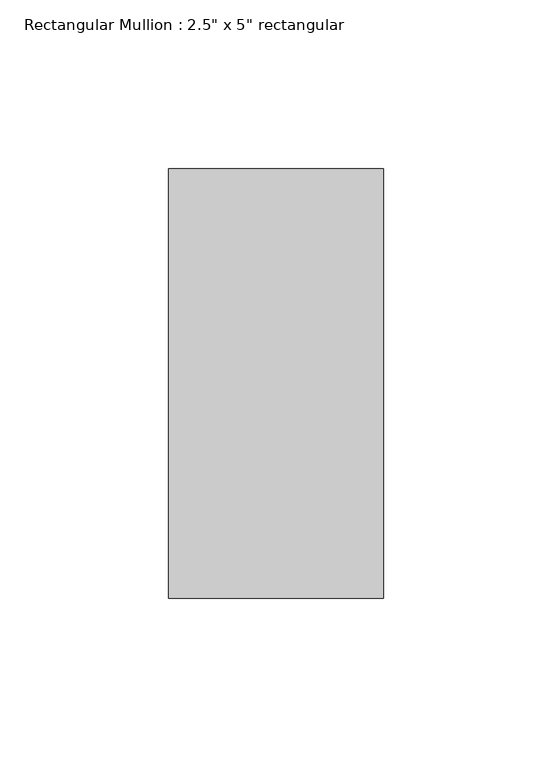
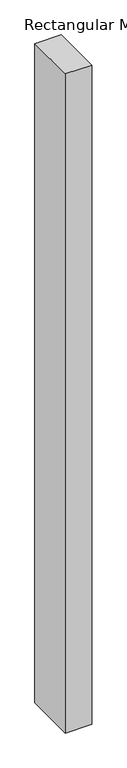
"""IFC4 building model written with IfcOpenShell, lengths in millimetres: member geometry."""

from ifc_helpers import new_model, si_unit, frame, origin, place, context, project, spatial, polyline, outline, extrude, source, transform, mapped, element, save


def member_d74592ed(model_context):
    return source(origin(), model_context, "Body", "SweptSolid", [
        extrude(outline(polyline([(31.75, 63.5), (31.75, -63.5), (-31.75, -63.5), (-31.75, 63.5), (31.75, 63.5)])), frame((0.0, 0.0, -1680.4980219), z_axis=(0.0, 0.0, 1.0), x_axis=(1.0, 0.0, 0.0)), (0.0, 0.0, 1.0), 1680.4980219),
    ])


if __name__ == "__main__":
    model = new_model("IFC4")
    model_context = context("Model", 3, world=origin())
    ifc_project = project(units=[si_unit("LENGTHUNIT", "METRE", prefix="MILLI")], contexts=[model_context])
    site = spatial("IfcSite", under=ifc_project)
    building = spatial("IfcBuilding", under=site)
    placement = place(None, origin())
    member_shape = member_d74592ed(model_context)
    element("IfcMember", 1, ObjectType="Rectangular Mullion : 2.5\" x 5\" rectangular", at=placement, inside=building, context=model_context, shape_type="MappedRepresentation", body=[
        mapped(member_shape, transform((0.0, 0.0, 0.0), x_axis=(1.0, 0.0, 0.0), y_axis=(0.0, 1.0, 0.0), z_axis=(0.0, 0.0, 1.0))),
    ])
    save(model, "model.ifc")

# Revit data of these elements
# Type "Rectangular Mullion : 2.5\" x 5\" rectangular"
#   built-in parameter 1007304 = 0.416667 (stored number, unit not read)
#   built-in parameter 1007301 = 0.104167 (stored number, unit not read)
#   built-in parameter 1007300 = 0.104167 (stored number, unit not read)
# Element 1 (IfcMember, "Rectangular Mullion : 2.5\" x 5\" rectangular")
#   Materials on its faces: "Aluminum"
# Materials
#   "Aluminum": class "Metal", colour RGB 247 247 247, transparency 0, Description = "Aluminum 6061", Cost = 0
